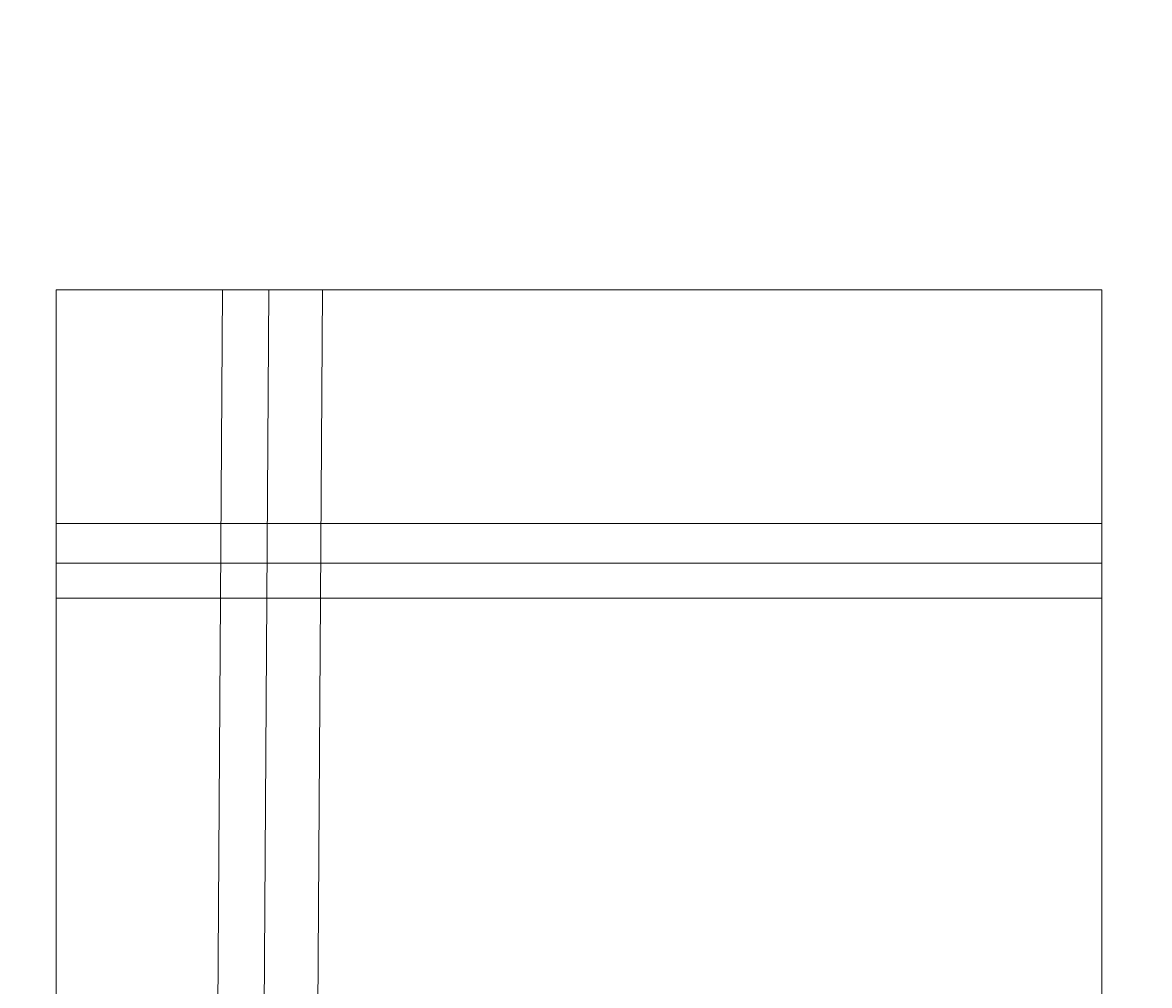
# Model space of a CAD drawing. Units: inches. Extents: x -46 to 1145, y -527 to 760.
# Tile 30 of 57: x 47 to 111, y 277 to 332. Entities that reach past the tile are written whole.
import ezdxf

# ---------------------------------------------------------------- set-up
doc = ezdxf.new("R2010")
doc.units = ezdxf.units.IN
doc.header["$MEASUREMENT"] = 0
doc.layers.add('A-ANNO-DIMS', color=2, linetype='Continuous', lineweight=18)
doc.layers.add('A-FURN', color=2, linetype='Continuous', lineweight=13)
doc.styles.get("Standard").update_dxf_attribs({"font": 'arial.ttf'})
doc.dimstyles.get("Standard").update_dxf_attribs({"dimtxt": 0.18, "dimasz": 0.18, "dimexe": 0.18, "dimexo": 0.0625, "dimgap": 0.09, "dimtad": 0, "dimtih": 1, "dimtoh": 1, "dimdec": 0, "dimzin": 0, "dimdsep": 46, "dimlunit": 3, "dimtxsty": 'Standard', "dimcen": 0.09, "dimadec": 0, "dimazin": 0, "dimtfac": 1, "dimtdec": 0, "dimtofl": 0, "dimtmove": 0, "dimatfit": 3, "dimfxl": 1, "dimtolj": 1, "dimtzin": 0, "dimarcsym": 0})

# ---------------------------------------------------------------- blocks, each defined once
blk = doc.blocks.new('BED-QUEEN-FURNISHED')
for p, q in [((0, 0), (0, 80)), ((60, 80), (60, 0)), ((44.724, 0), (45.016, 45.372)), ((47.804, 0), (48.097, 45.499)), ((50.463, 0), (50.758, 45.907)), ((0, 17.701), (60, 17.701)), ((0, 15.692), (60, 15.692)), ((0, 13.416), (60, 13.416)), ((60, 0), (0, 0))]:
    blk.add_line(p, q)
blk = doc.blocks.new('*D685')
at = {"layer": 'A-ANNO-DIMS', "color": 0, "lineweight": -2, "transparency": 16777216}
for p, q in [((183.501, 700.889), (-46.216, 700.889)), ((-46.036, 700.709), (-46.036, 116.385)), ((-46.036, -468.302), (-46.036, 116.021)), ((12.501, -468.482), (-46.216, -468.482))]:
    blk.add_line(p, q, dxfattribs=at)
at = {"layer": 'A-ANNO-DIMS', "color": 0, "transparency": 16777216}
for points in [[(-46.066, 700.709), (-46.006, 700.709), (-46.036, 700.889)], [(-46.066, -468.302), (-46.006, -468.302), (-46.036, -468.482)]]:
    blk.add_solid(points, dxfattribs=at)
at = {"layer": 'Defpoints', "color": 0, "transparency": 16777216}
for p in [(-46.036, 700.889), (183.564, 700.889), (12.564, -468.482)]:
    blk.add_point(p, dxfattribs=at)
at = {"layer": 'A-ANNO-DIMS', "color": 0, "transparency": 16777216, "insert": (-46.036, 116.203), "char_height": 0.18, "attachment_point": 5}
blk.add_mtext('\\A1;1169.4', dxfattribs=at)

msp = doc.modelspace()

# ---------------------------------------------------------------- block references
at = {"layer": 'A-FURN', "rotation": 180}
msp.add_blockref('BED-QUEEN-FURNISHED', (108.4877, 316.6818), dxfattribs=at)

# ---------------------------------------------------------------- dimensions: what is measured, and where the dimension line sits
at = {"layer": 'A-ANNO-DIMS'}
dim = msp.add_linear_dim(base=(-46.0363, 700.8886), p1=(12.5637, -468.4824), p2=(183.5637, 700.8886), angle=90, dimstyle='Standard', override={"dimdec": 1, "dimlfac": 1, "dimrnd": 0, "dimzin": 0, "dimdsep": 46, "dimlunit": 2}, dxfattribs=at)
dim.commit()
dim.dimension.update_dxf_attribs({"geometry": '*D685', "text_midpoint": (-46.0363, 116.2031)})

doc.saveas('drawing.dxf')
